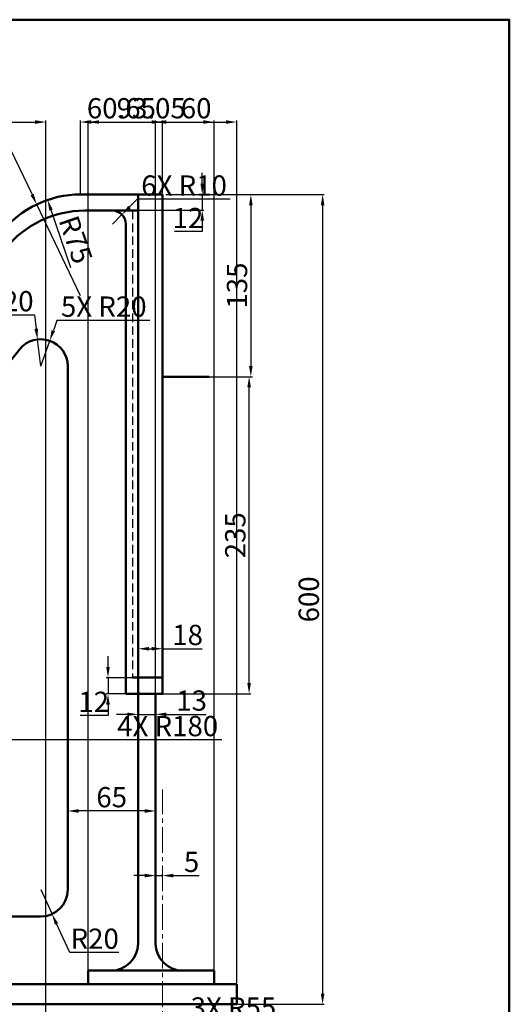
# Model space of a CAD drawing. Units: millimetres. Extents: x -60 to 1204, y -103 to 1006.
# Tile 4 of 4: x 842 to 1204, y 277 to 1006. Entities that reach past the tile are written whole.
import ezdxf

# ---------------------------------------------------------------- set-up
doc = ezdxf.new("R2010")
doc.units = ezdxf.units.MM
doc.linetypes.add('CENTER2', pattern=[28.575, 19.05, -3.175, 3.175, -3.175])
doc.linetypes.add('DASHED', pattern=[19.05, 12.7, -6.35])
for name, color, linetype, lineweight in [('M-CNTR', 1, 'CENTER2', 18), ('M-DIMS', 2, 'Continuous', 25), ('M-HIDN', 4, 'DASHED', 25), ('M-OUTL', 7, 'Continuous', 50), ('M-TTLB', 7, 'Continuous', 50)]:
    doc.layers.add(name, color=color, linetype=linetype, lineweight=lineweight)
doc.styles.get("Standard").update_dxf_attribs({"font": 'arial.ttf'})
doc.dimstyles.new('ISO-25', dxfattribs={"dimtxt": 15, "dimasz": 8, "dimexe": 1.25, "dimexo": 0.625, "dimtad": 1, "dimtoh": 1, "dimdec": 0, "dimtxsty": 'Standard', "dimcen": 2.5, "dimadec": 0, "dimazin": 0, "dimtfac": 1, "dimtdec": 0, "dimtmove": 0, "dimatfit": 3, "dimfxl": 1, "dimarcsym": 0})

# ---------------------------------------------------------------- blocks, each defined once
blk = doc.blocks.new('*U2')
at = {"layer": 'M-CNTR', "color": 0, "transparency": 16777216}
for p, q in [((0, 11), (0, 257.93)), ((-58.5, 0), (-11, 0)), ((11, 0), (58.5, 0)), ((0, -58.5), (0, -11))]:
    blk.add_line(p, q, dxfattribs=at)
at = {"layer": 'M-CNTR', "color": 0, "linetype": 'Continuous', "transparency": 16777216}
for p, q in [((-5.5, 0), (5.5, 0)), ((0, -5.5), (0, 5.5))]:
    blk.add_line(p, q, dxfattribs=at)
blk = doc.blocks.new('*U4')
at = {"layer": 'M-CNTR', "color": 0, "transparency": 16777216}
blk.add_line((-32.4, 0), (154.61, 0), dxfattribs=at)
blk = doc.blocks.new('*D36')
at = {"layer": 'Defpoints', "color": 0, "transparency": 16777216}
for p in [(929.53, 490.14), (942.53, 491.48), (942.53, 490.14)]:
    blk.add_point(p, dxfattribs=at)
at = {"layer": 'M-DIMS', "color": 0, "lineweight": -2, "transparency": 16777216}
for p, q in [((921.53, 491.48), (913.53, 491.48)), ((929.53, 490.76), (929.53, 492.73)), ((929.53, 491.48), (942.53, 491.48)), ((942.53, 490.76), (942.53, 492.73)), ((950.53, 491.48), (979.86, 491.48))]:
    blk.add_line(p, q, dxfattribs=at)
at = {"layer": 'M-DIMS', "color": 0, "transparency": 16777216}
for points in [[(921.53, 492.82), (921.53, 490.15), (929.53, 491.48)], [(950.53, 492.82), (950.53, 490.15), (942.53, 491.48)]]:
    blk.add_solid(points, dxfattribs=at)
at = {"layer": 'M-DIMS', "color": 0, "transparency": 16777216, "insert": (969.19, 499.77), "char_height": 15, "attachment_point": 5}
blk.add_mtext('13', dxfattribs=at)
blk = doc.blocks.new('*D37')
at = {"layer": 'Defpoints', "color": 0, "transparency": 16777216}
for p in [(877.53, 419.9), (942.53, 414.16), (877.53, 399.16)]:
    blk.add_point(p, dxfattribs=at)
at = {"layer": 'M-DIMS', "color": 0, "lineweight": -2, "transparency": 16777216}
for p, q in [((877.53, 399.79), (877.53, 421.15)), ((934.53, 419.9), (885.53, 419.9)), ((942.53, 414.79), (942.53, 421.15))]:
    blk.add_line(p, q, dxfattribs=at)
at = {"layer": 'M-DIMS', "color": 0, "transparency": 16777216}
for points in [[(885.53, 421.23), (885.53, 418.56), (877.53, 419.9)], [(934.53, 421.23), (934.53, 418.56), (942.53, 419.9)]]:
    blk.add_solid(points, dxfattribs=at)
at = {"layer": 'M-DIMS', "color": 0, "transparency": 16777216, "insert": (910.03, 428.18), "char_height": 15, "attachment_point": 5}
blk.add_mtext('65', dxfattribs=at)
blk = doc.blocks.new('*D38')
at = {"layer": 'Defpoints', "color": 0, "transparency": 16777216}
for p in [(942.53, 370.67), (947.53, 372.01), (947.53, 370.67)]:
    blk.add_point(p, dxfattribs=at)
at = {"layer": 'M-DIMS', "color": 0, "lineweight": -2, "transparency": 16777216}
for p, q in [((942.53, 371.29), (942.53, 373.26)), ((947.53, 371.29), (947.53, 373.26)), ((934.53, 372.01), (926.53, 372.01)), ((942.53, 372.01), (947.53, 372.01)), ((955.53, 372.01), (974.73, 372.01))]:
    blk.add_line(p, q, dxfattribs=at)
at = {"layer": 'M-DIMS', "color": 0, "transparency": 16777216}
for points in [[(934.53, 373.34), (934.53, 370.68), (942.53, 372.01)], [(955.53, 373.34), (955.53, 370.68), (947.53, 372.01)]]:
    blk.add_solid(points, dxfattribs=at)
at = {"layer": 'M-DIMS', "color": 0, "transparency": 16777216, "insert": (969.13, 380.26), "char_height": 15, "attachment_point": 5}
blk.add_mtext('5', dxfattribs=at)
blk = doc.blocks.new('*D39')
at = {"layer": 'Defpoints', "color": 0, "transparency": 16777216}
for p in [(949.51, 876.66), (1002.53, 276.66), (1066.11, 276.66)]:
    blk.add_point(p, dxfattribs=at)
at = {"layer": 'M-DIMS', "color": 0, "lineweight": -2, "transparency": 16777216}
for p, q in [((950.13, 876.66), (1067.36, 876.66)), ((1066.11, 868.66), (1066.11, 284.66)), ((1003.16, 276.66), (1067.36, 276.66))]:
    blk.add_line(p, q, dxfattribs=at)
at = {"layer": 'M-DIMS', "color": 0, "transparency": 16777216}
for points in [[(1064.78, 868.66), (1067.45, 868.66), (1066.11, 876.66)], [(1064.78, 284.66), (1067.45, 284.66), (1066.11, 276.66)]]:
    blk.add_solid(points, dxfattribs=at)
at = {"layer": 'M-DIMS', "color": 0, "transparency": 16777216, "insert": (1057.83, 576.66), "char_height": 15, "attachment_point": 5, "rotation": 90}
blk.add_mtext('600', dxfattribs=at)
blk = doc.blocks.new('*D40')
at = {"layer": 'Defpoints', "color": 0, "transparency": 16777216}
for p in [(929.53, 518.66), (907.3, 506.66), (929.53, 506.66)]:
    blk.add_point(p, dxfattribs=at)
at = {"layer": 'M-DIMS', "color": 0, "lineweight": -2, "transparency": 16777216}
for p, q in [((907.3, 526.66), (907.3, 534.66)), ((928.91, 518.66), (906.05, 518.66)), ((907.3, 518.66), (907.3, 506.66)), ((928.91, 506.66), (906.05, 506.66)), ((907.3, 498.66), (907.3, 490.66)), ((907.3, 490.66), (886.75, 490.66))]:
    blk.add_line(p, q, dxfattribs=at)
at = {"layer": 'M-DIMS', "color": 0, "transparency": 16777216}
for points in [[(905.96, 526.66), (908.63, 526.66), (907.3, 518.66)], [(905.96, 498.66), (908.63, 498.66), (907.3, 506.66)]]:
    blk.add_solid(points, dxfattribs=at)
at = {"layer": 'M-DIMS', "color": 0, "transparency": 16777216, "insert": (896.71, 498.82), "char_height": 15, "attachment_point": 5}
blk.add_mtext('12', dxfattribs=at)
blk = doc.blocks.new('*D41')
at = {"layer": 'Defpoints', "color": 0, "transparency": 16777216}
for p in [(947.53, 540.09), (929.53, 538.91), (947.53, 538.91)]:
    blk.add_point(p, dxfattribs=at)
at = {"layer": 'M-DIMS', "color": 0, "lineweight": -2, "transparency": 16777216}
for p, q in [((929.53, 539.53), (929.53, 541.34)), ((937.53, 540.09), (939.53, 540.09)), ((947.53, 539.53), (947.53, 541.34)), ((947.53, 540.09), (976.89, 540.09))]:
    blk.add_line(p, q, dxfattribs=at)
at = {"layer": 'M-DIMS', "color": 0, "transparency": 16777216}
for points in [[(937.53, 541.42), (937.53, 538.76), (929.53, 540.09)], [(939.53, 541.42), (939.53, 538.76), (947.53, 540.09)]]:
    blk.add_solid(points, dxfattribs=at)
at = {"layer": 'M-DIMS', "color": 0, "transparency": 16777216, "insert": (966.21, 548.38), "char_height": 15, "attachment_point": 5}
blk.add_mtext('18', dxfattribs=at)
blk = doc.blocks.new('*D42')
at = {"layer": 'Defpoints', "color": 0, "transparency": 16777216}
for p in [(954.61, 876.66), (964.83, 741.66), (1013.01, 741.66)]:
    blk.add_point(p, dxfattribs=at)
at = {"layer": 'M-DIMS', "color": 0, "lineweight": -2, "transparency": 16777216}
for p, q in [((955.23, 876.66), (1014.26, 876.66)), ((1013.01, 868.66), (1013.01, 749.66)), ((965.45, 741.66), (1014.26, 741.66))]:
    blk.add_line(p, q, dxfattribs=at)
at = {"layer": 'M-DIMS', "color": 0, "transparency": 16777216}
for points in [[(1011.67, 868.66), (1014.34, 868.66), (1013.01, 876.66)], [(1011.67, 749.66), (1014.34, 749.66), (1013.01, 741.66)]]:
    blk.add_solid(points, dxfattribs=at)
at = {"layer": 'M-DIMS', "color": 0, "transparency": 16777216, "insert": (1004.72, 809.16), "char_height": 15, "attachment_point": 5, "rotation": 90}
blk.add_mtext('135', dxfattribs=at)
blk = doc.blocks.new('*D43')
at = {"layer": 'Defpoints', "color": 0, "transparency": 16777216}
for p in [(964.83, 741.66), (1011.71, 741.66), (942.53, 506.66)]:
    blk.add_point(p, dxfattribs=at)
at = {"layer": 'M-DIMS', "color": 0, "lineweight": -2, "transparency": 16777216}
for p, q in [((965.45, 741.66), (1012.96, 741.66)), ((1011.71, 514.66), (1011.71, 733.66)), ((943.16, 506.66), (1012.96, 506.66))]:
    blk.add_line(p, q, dxfattribs=at)
at = {"layer": 'M-DIMS', "color": 0, "transparency": 16777216}
for points in [[(1010.37, 733.66), (1013.04, 733.66), (1011.71, 741.66)], [(1010.37, 514.66), (1013.04, 514.66), (1011.71, 506.66)]]:
    blk.add_solid(points, dxfattribs=at)
at = {"layer": 'M-DIMS', "color": 0, "transparency": 16777216, "insert": (1003.42, 624.16), "char_height": 15, "attachment_point": 5, "rotation": 90}
blk.add_mtext('235', dxfattribs=at)
blk = doc.blocks.new('*D44')
at = {"layer": 'Defpoints', "color": 0, "transparency": 16777216}
for p in [(949.51, 876.66), (929.53, 865.13), (977.03, 865.13)]:
    blk.add_point(p, dxfattribs=at)
at = {"layer": 'M-DIMS', "color": 0, "lineweight": -2, "transparency": 16777216}
for p, q in [((977.03, 884.66), (977.03, 892.66)), ((950.13, 876.66), (978.28, 876.66)), ((977.03, 876.66), (977.03, 865.13)), ((930.16, 865.13), (978.28, 865.13)), ((977.03, 857.13), (977.03, 849.13)), ((977.03, 849.13), (956.48, 849.13))]:
    blk.add_line(p, q, dxfattribs=at)
at = {"layer": 'M-DIMS', "color": 0, "transparency": 16777216}
for points in [[(975.69, 884.66), (978.36, 884.66), (977.03, 876.66)], [(975.69, 857.13), (978.36, 857.13), (977.03, 865.13)]]:
    blk.add_solid(points, dxfattribs=at)
at = {"layer": 'M-DIMS', "color": 0, "transparency": 16777216, "insert": (966.44, 857.29), "char_height": 15, "attachment_point": 5}
blk.add_mtext('12', dxfattribs=at)
blk = doc.blocks.new('*D45')
at = {"layer": 'Defpoints', "color": 0, "transparency": 16777216}
for p in [(862.58, 872.62), (886.88, 801.66)]:
    blk.add_point(p, dxfattribs=at)
at = {"layer": 'M-DIMS', "color": 0, "lineweight": -2, "transparency": 16777216}
blk.add_line((879.82, 822.28), (865.17, 865.05), dxfattribs=at)
at = {"layer": 'M-DIMS', "color": 0, "transparency": 16777216}
blk.add_solid([(866.43, 865.48), (863.91, 864.62), (862.58, 872.62)], dxfattribs=at)
at = {"layer": 'M-DIMS', "color": 0, "transparency": 16777216, "insert": (881.6, 842.56), "char_height": 15, "attachment_point": 5, "rotation": 288.90618}
blk.add_mtext('R75', dxfattribs=at)
blk = doc.blocks.new('*D46')
at = {"layer": 'Defpoints', "color": 0, "transparency": 16777216}
for p in [(855.11, 769.26), (857.53, 749.41)]:
    blk.add_point(p, dxfattribs=at)
at = {"layer": 'M-DIMS', "color": 0, "lineweight": -2, "transparency": 16777216}
for p, q in [((816.49, 787.37), (852.9, 787.37)), ((852.9, 787.37), (854.14, 777.2)), ((857.53, 749.41), (855.11, 769.26))]:
    blk.add_line(p, q, dxfattribs=at)
at = {"layer": 'M-DIMS', "color": 0, "transparency": 16777216}
blk.add_solid([(855.47, 777.36), (852.82, 777.04), (855.11, 769.26)], dxfattribs=at)
at = {"layer": 'M-DIMS', "color": 0, "transparency": 16777216, "insert": (834.38, 795.65), "char_height": 15, "attachment_point": 5}
blk.add_mtext('R20', dxfattribs=at)
blk = doc.blocks.new('*D48')
at = {"layer": 'Defpoints', "color": 0, "transparency": 16777216}
for p in [(857.53, 361.66), (865.88, 343.49)]:
    blk.add_point(p, dxfattribs=at)
at = {"layer": 'M-DIMS', "color": 0, "lineweight": -2, "transparency": 16777216}
for p, q in [((857.53, 361.66), (865.88, 343.49)), ((878.95, 315.03), (869.22, 336.22)), ((915.37, 315.03), (878.95, 315.03))]:
    blk.add_line(p, q, dxfattribs=at)
at = {"layer": 'M-DIMS', "color": 0, "transparency": 16777216}
blk.add_solid([(870.43, 336.78), (868.01, 335.66), (865.88, 343.49)], dxfattribs=at)
at = {"layer": 'M-DIMS', "color": 0, "transparency": 16777216, "insert": (897.48, 323.32), "char_height": 15, "attachment_point": 5}
blk.add_mtext('R20', dxfattribs=at)
blk = doc.blocks.new('*D62')
at = {"layer": 'Defpoints', "color": 0, "transparency": 16777216}
for p in [(1002.53, 930.31), (942.53, 321.66), (1002.53, 291.66)]:
    blk.add_point(p, dxfattribs=at)
at = {"layer": 'M-DIMS', "color": 0, "lineweight": -2, "transparency": 16777216}
for p, q in [((942.53, 322.29), (942.53, 931.56)), ((950.53, 930.31), (994.53, 930.31)), ((1002.53, 292.29), (1002.53, 931.56))]:
    blk.add_line(p, q, dxfattribs=at)
at = {"layer": 'M-DIMS', "color": 0, "transparency": 16777216}
for points in [[(950.53, 931.65), (950.53, 928.98), (942.53, 930.31)], [(994.53, 931.65), (994.53, 928.98), (1002.53, 930.31)]]:
    blk.add_solid(points, dxfattribs=at)
at = {"layer": 'M-DIMS', "color": 0, "transparency": 16777216, "insert": (972.53, 938.6), "char_height": 15, "attachment_point": 5}
blk.add_mtext('60', dxfattribs=at)
blk = doc.blocks.new('*D65')
at = {"layer": 'Defpoints', "color": 0, "transparency": 16777216}
for p in [(985.78, 930.31), (892.73, 301.66), (985.78, 301.66)]:
    blk.add_point(p, dxfattribs=at)
at = {"layer": 'M-DIMS', "color": 0, "lineweight": -2, "transparency": 16777216}
for p, q in [((892.73, 302.29), (892.73, 931.56)), ((900.73, 930.31), (977.78, 930.31)), ((985.78, 302.29), (985.78, 931.56))]:
    blk.add_line(p, q, dxfattribs=at)
at = {"layer": 'M-DIMS', "color": 0, "transparency": 16777216}
for points in [[(900.73, 931.65), (900.73, 928.98), (892.73, 930.31)], [(977.78, 931.65), (977.78, 928.98), (985.78, 930.31)]]:
    blk.add_solid(points, dxfattribs=at)
at = {"layer": 'M-DIMS', "color": 0, "transparency": 16777216, "insert": (939.26, 938.6), "char_height": 15, "attachment_point": 5}
blk.add_mtext('93.05', dxfattribs=at)
blk = doc.blocks.new('*D66')
at = {"layer": 'Defpoints', "color": 0, "transparency": 16777216}
for p in [(947.53, 930.31), (886.88, 876.66), (947.53, 876.66)]:
    blk.add_point(p, dxfattribs=at)
at = {"layer": 'M-DIMS', "color": 0, "lineweight": -2, "transparency": 16777216}
for p, q in [((886.88, 877.29), (886.88, 931.56)), ((894.88, 930.31), (939.53, 930.31)), ((947.53, 877.29), (947.53, 931.56))]:
    blk.add_line(p, q, dxfattribs=at)
at = {"layer": 'M-DIMS', "color": 0, "transparency": 16777216}
for points in [[(894.88, 931.65), (894.88, 928.98), (886.88, 930.31)], [(939.53, 931.65), (939.53, 928.98), (947.53, 930.31)]]:
    blk.add_solid(points, dxfattribs=at)
at = {"layer": 'M-DIMS', "color": 0, "transparency": 16777216, "insert": (917.21, 938.6), "char_height": 15, "attachment_point": 5}
blk.add_mtext('60.65', dxfattribs=at)
blk = doc.blocks.new('*D68')
at = {"layer": 'Defpoints', "color": 0, "transparency": 16777216}
for p in [(861.39, 930.31), (861.39, 175.77), (347.53, 107.92)]:
    blk.add_point(p, dxfattribs=at)
at = {"layer": 'M-DIMS', "color": 0, "lineweight": -2, "transparency": 16777216}
for p, q in [((347.53, 108.55), (347.53, 931.56)), ((355.53, 930.31), (853.39, 930.31)), ((861.39, 176.39), (861.39, 931.56))]:
    blk.add_line(p, q, dxfattribs=at)
at = {"layer": 'M-DIMS', "color": 0, "transparency": 16777216}
for points in [[(355.53, 931.65), (355.53, 928.98), (347.53, 930.31)], [(853.39, 931.65), (853.39, 928.98), (861.39, 930.31)]]:
    blk.add_solid(points, dxfattribs=at)
at = {"layer": 'M-DIMS', "color": 0, "transparency": 16777216, "insert": (604.46, 938.6), "char_height": 15, "attachment_point": 5}
blk.add_mtext('513.9', dxfattribs=at)
blk = doc.blocks.new('*D70')
at = {"layer": 'Defpoints', "color": 0, "transparency": 16777216}
for p in [(622.67, 472.57), (802.67, 472.57)]:
    blk.add_point(p, dxfattribs=at)
at = {"layer": 'M-DIMS', "color": 0, "lineweight": -2, "transparency": 16777216}
for p, q in [((622.67, 472.57), (802.67, 472.57)), ((910.67, 472.57), (810.67, 472.57)), ((991.58, 472.57), (910.67, 472.57))]:
    blk.add_line(p, q, dxfattribs=at)
at = {"layer": 'M-DIMS', "color": 0, "transparency": 16777216}
blk.add_solid([(810.67, 473.9), (810.67, 471.24), (802.67, 472.57)], dxfattribs=at)
at = {"layer": 'M-DIMS', "color": 0, "transparency": 16777216, "insert": (951.44, 480.85), "char_height": 15, "attachment_point": 5}
blk.add_mtext('4X R180', dxfattribs=at)
blk = doc.blocks.new('*D72')
at = {"layer": 'Defpoints', "color": 0, "transparency": 16777216}
for p in [(854.55, 869.34), (886.88, 801.66)]:
    blk.add_point(p, dxfattribs=at)
at = {"layer": 'M-DIMS', "color": 0, "lineweight": -2, "transparency": 16777216}
for p, q in [((766.08, 909.94), (835.15, 909.94)), ((835.15, 909.94), (851.1, 876.56)), ((886.88, 801.66), (854.55, 869.34))]:
    blk.add_line(p, q, dxfattribs=at)
at = {"layer": 'M-DIMS', "color": 0, "transparency": 16777216}
blk.add_solid([(852.3, 877.13), (849.9, 875.98), (854.55, 869.34)], dxfattribs=at)
at = {"layer": 'M-DIMS', "color": 0, "transparency": 16777216, "insert": (800.3, 918.22), "char_height": 15, "attachment_point": 5}
blk.add_mtext('2X R75', dxfattribs=at)
blk = doc.blocks.new('*D73')
at = {"layer": 'Defpoints', "color": 0, "transparency": 16777216}
for p in [(958.72, 231.77), (947.53, 177.92)]:
    blk.add_point(p, dxfattribs=at)
at = {"layer": 'M-DIMS', "color": 0, "lineweight": -2, "transparency": 16777216}
for p, q in [((965.43, 264.08), (960.34, 239.6)), ((1034.23, 264.08), (965.43, 264.08)), ((947.53, 177.92), (958.72, 231.77))]:
    blk.add_line(p, q, dxfattribs=at)
at = {"layer": 'M-DIMS', "color": 0, "transparency": 16777216}
blk.add_solid([(959.04, 239.87), (961.65, 239.33), (958.72, 231.77)], dxfattribs=at)
at = {"layer": 'M-DIMS', "color": 0, "transparency": 16777216, "insert": (1000.14, 272.37), "char_height": 15, "attachment_point": 5}
blk.add_mtext('3X R55', dxfattribs=at)
blk = doc.blocks.new('*D76')
at = {"layer": 'Defpoints', "color": 0, "transparency": 16777216}
for p in [(864.19, 768.26), (857.53, 749.41)]:
    blk.add_point(p, dxfattribs=at)
at = {"layer": 'M-DIMS', "color": 0, "lineweight": -2, "transparency": 16777216}
for p, q in [((869.52, 783.35), (866.86, 775.81)), ((938.17, 783.35), (869.52, 783.35)), ((857.53, 749.41), (864.19, 768.26))]:
    blk.add_line(p, q, dxfattribs=at)
at = {"layer": 'M-DIMS', "color": 0, "transparency": 16777216}
blk.add_solid([(865.6, 776.25), (868.12, 775.36), (864.19, 768.26)], dxfattribs=at)
at = {"layer": 'M-DIMS', "color": 0, "transparency": 16777216, "insert": (904.16, 791.63), "char_height": 15, "attachment_point": 5}
blk.add_mtext('5X R20', dxfattribs=at)
blk = doc.blocks.new('*D77')
at = {"layer": 'Defpoints', "color": 0, "transparency": 16777216}
for p in [(917.6, 861.74), (910.53, 854.66)]:
    blk.add_point(p, dxfattribs=at)
at = {"layer": 'M-DIMS', "color": 0, "lineweight": -2, "transparency": 16777216}
for p, q in [((928.92, 873.05), (923.26, 867.39)), ((997.64, 873.05), (928.92, 873.05)), ((910.53, 854.66), (917.6, 861.74))]:
    blk.add_line(p, q, dxfattribs=at)
at = {"layer": 'M-DIMS', "color": 0, "transparency": 16777216}
blk.add_solid([(922.32, 868.33), (924.2, 866.45), (917.6, 861.74)], dxfattribs=at)
at = {"layer": 'M-DIMS', "color": 0, "transparency": 16777216, "insert": (963.59, 881.33), "char_height": 15, "attachment_point": 5}
blk.add_mtext('6X R10', dxfattribs=at)

msp = doc.modelspace()

# ---------------------------------------------------------------- linework, layer by layer
at = {"layer": 'M-HIDN', "ltscale": 0.5}
msp.add_line((925.3879, 864.6642), (925.3879, 518.6642), dxfattribs=at)
at = {"layer": 'M-OUTL'}
for p, q in [((886.8808, 876.6642), (929.5307, 876.6642)), ((929.5307, 876.6642), (942.5307, 876.6642)), ((929.5307, 321.6642), (929.5307, 876.6642)), ((947.5307, 876.6642), (942.5307, 876.6642)), ((947.5307, 506.6642), (947.5307, 876.6642)), ((890.0435, 864.6642), (910.5307, 864.6642)), ((920.5307, 506.6642), (920.5307, 854.6642)), ((877.5307, 361.6642), (877.5307, 749.4057)), ((947.5307, 518.6642), (925.3879, 518.6642)), ((942.5307, 506.6642), (920.5307, 506.6642)), ((929.5307, 506.6642), (942.5307, 506.6642)), ((942.5307, 321.6642), (942.5307, 506.6642)), ((942.5307, 506.6642), (947.5307, 506.6642)), ((544.3907, 341.6642), (857.5307, 341.6642)), ((909.5307, 301.6642), (892.7335, 301.6642)), ((892.7335, 301.6642), (892.7335, 291.6642)), ((985.7804, 301.6642), (909.5307, 301.6642)), ((985.7804, 291.6642), (985.7804, 301.6642)), ((292.5307, 291.6642), (1002.5307, 291.6642)), ((947.5307, 291.6642), (942.5307, 291.6642)), ((1002.5307, 276.6642), (1002.5307, 291.6642)), ((292.5307, 276.6642), (1002.5307, 276.6642))]:
    msp.add_line(p, q, dxfattribs=at)
at = {"layer": 'M-OUTL', "ltscale": 0.5}
for p, q in [((910.5307, 864.6642), (929.5307, 864.6642)), ((528.8312, 374.2301), (841.9712, 761.9716)), ((947.5307, 741.6642), (982.1277, 741.6642))]:
    msp.add_line(p, q, dxfattribs=at)
for centre in [(886.8808, 801.6642), (890.0435, 789.6642)]:
    msp.add_arc(centre, 75, 90, 141.0756607, dxfattribs=at)
at = {"layer": 'M-OUTL'}
for centre, radius, start, end in [((910.5307, 854.6642), 10, 0, 90), ((857.5307, 749.4057), 20, 0, 141.0756607), ((857.5307, 361.6642), 20, 270, 0), ((909.5307, 321.6642), 20, 270, 0), ((962.5307, 321.6642), 20, 180, 270)]:
    msp.add_arc(centre, radius, start, end, dxfattribs=at)
at = {"layer": 'M-TTLB'}
msp.add_lwpolyline([(-59.5454, 1006.1383), (1204.2342, 1006.1383), (1204.2342, -103.2116), (-59.5454, -103.2116)], close=True, dxfattribs=at)

# ---------------------------------------------------------------- block references
at = {"layer": 'M-CNTR'}
for name, p in [('*U4', (753.1727, 472.5699)), ('*U2', (947.5307, 177.9202))]:
    msp.add_blockref(name, p, dxfattribs=at)

# ---------------------------------------------------------------- dimensions: what is measured, and where the dimension line sits
at = {"layer": 'M-DIMS'}
for base, p1, p2, override, picture, middle in [((861.3892, 930.3142), (347.5307, 107.9202), (861.3892, 175.7691), {"dimdec": 1, "dimlfac": 1, "dimrnd": 0, "dimzin": 0, "dimdsep": 46, "dimlunit": 2}, '*D68', (604.46, 938.6029)), ((947.5307, 930.3142), (886.8808, 876.6642), (947.5307, 876.6642), {"dimdec": 2, "dimlfac": 1, "dimrnd": 0, "dimzin": 0, "dimdsep": 46, "dimlunit": 2}, '*D66', (917.2058, 938.5978)), ((985.7804, 930.3142), (892.7335, 301.6642), (985.7804, 301.6642), {"dimdec": 2, "dimlfac": 1, "dimrnd": 0, "dimzin": 0, "dimdsep": 46, "dimlunit": 2}, '*D65', (939.2569, 938.6029)), ((1002.5307, 930.3142), (942.5307, 321.6642), (1002.5307, 291.6642), {"dimdec": 0, "dimlfac": 1, "dimrnd": 0, "dimzin": 0, "dimdsep": 46, "dimlunit": 2}, '*D62', (972.5307, 938.5978)), ((947.5307, 540.0915), (929.5307, 538.9056), (947.5307, 538.9056), {"dimclrd": 0, "dimclre": 0, "dimclrt": 0}, '*D41', (966.2086, 548.3751)), ((942.5307, 491.4836), (929.5307, 490.1389), (942.5307, 490.1389), {"dimclrd": 0, "dimclre": 0, "dimclrt": 0}, '*D36', (969.1933, 499.7723)), ((877.5307, 419.8975), (942.5307, 414.1642), (877.5307, 399.1642), {"dimclrd": 0, "dimclre": 0, "dimclrt": 0}, '*D37', (910.0307, 428.1811)), ((947.5307, 372.0108), (942.5307, 370.6661), (947.5307, 370.6661), {"dimclrd": 0, "dimclre": 0, "dimclrt": 0}, '*D38', (969.1285, 380.2637))]:
    dim = msp.add_linear_dim(base=base, p1=p1, p2=p2, dimstyle='ISO-25', override=override, dxfattribs=at)
    dim.commit()
    dim.dimension.update_dxf_attribs({"geometry": picture, "text_midpoint": middle})
for center, mpoint, text, picture, middle in [((886.8808, 801.6642), (854.5481, 869.3369), '2X <>', '*D72', (800.3027, 909.9405)), ((622.6727, 472.5699), (802.6727, 472.57), '4X <>', '*D70', (910.6727, 472.57)), ((947.5307, 177.9202), (958.7169, 231.7706), '3X <>', '*D73', (1000.1413, 264.0809))]:
    dim = msp.add_radius_dim(center=center, mpoint=mpoint, text=text, dimstyle='ISO-25', override={"dimdec": 0, "dimlfac": 1, "dimrnd": 0, "dimzin": 0, "dimdsep": 46, "dimlunit": 2}, dxfattribs=at)
    dim.commit()
    dim.dimension.update_dxf_attribs({"geometry": picture, "text_midpoint": middle, "dimtype": 164})
for center, mpoint, text, picture, middle in [((910.5307, 854.6642), (917.602, 861.735), '6X <>', '*D77', (963.5929, 881.332)), ((857.5307, 749.4057), (864.194, 768.2631), '5X <>', '*D76', (904.1606, 791.6326))]:
    dim = msp.add_radius_dim(center=center, mpoint=mpoint, text=text, dimstyle='ISO-25', override={"dimdec": 0, "dimlfac": 1, "dimrnd": 0, "dimzin": 0, "dimdsep": 46, "dimlunit": 2}, dxfattribs=at)
    dim.commit()
    dim.dimension.update_dxf_attribs({"geometry": picture, "text_midpoint": middle})
for base, p1, p2, picture, middle in [((977.0281, 865.1301), (949.5083, 876.6642), (929.5307, 865.1301), '*D44', (966.4423, 857.2858)), ((1066.112, 276.6642), (949.5083, 876.6642), (1002.5307, 276.6642), '*D39', (1057.8284, 576.6642)), ((1013.0076, 741.6642), (954.6068, 876.6642), (964.8292, 741.6642), '*D42', (1004.7189, 809.1642)), ((1011.7055, 741.6642), (942.5307, 506.6642), (964.8292, 741.6642), '*D43', (1003.4168, 624.1642)), ((907.2974, 506.6642), (929.5307, 518.6642), (929.5307, 506.6642), '*D40', (896.7117, 498.8199))]:
    dim = msp.add_linear_dim(base=base, p1=p1, p2=p2, angle=90, dimstyle='ISO-25', override={"dimclrd": 0, "dimclre": 0, "dimclrt": 0}, dxfattribs=at)
    dim.commit()
    dim.dimension.update_dxf_attribs({"geometry": picture, "text_midpoint": middle})
for center, mpoint, picture, middle in [((886.8808, 801.6642), (862.5793, 872.618), '*D45', (873.7912, 839.8823)), ((857.5307, 749.4057), (855.1116, 769.2589), '*D46', (834.3841, 787.3695))]:
    dim = msp.add_radius_dim(center=center, mpoint=mpoint, dimstyle='ISO-25', override={"dimclrd": 0, "dimclre": 0, "dimclrt": 0}, dxfattribs=at)
    dim.commit()
    dim.dimension.update_dxf_attribs({"geometry": picture, "text_midpoint": middle, "dimtype": 164})
dim = msp.add_radius_dim(center=(857.5307, 361.6642), mpoint=(865.8804, 343.4905), dimstyle='ISO-25', override={"dimclrd": 0, "dimclre": 0, "dimclrt": 0}, dxfattribs=at)
dim.commit()
dim.dimension.update_dxf_attribs({"geometry": '*D48', "text_midpoint": (897.4753, 323.3166)})

doc.saveas('drawing.dxf')
